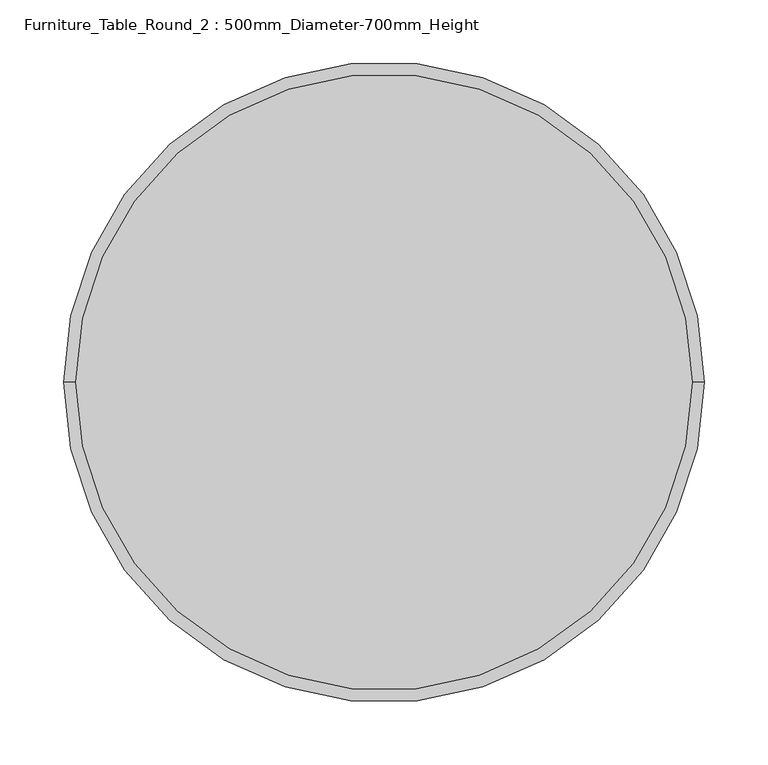
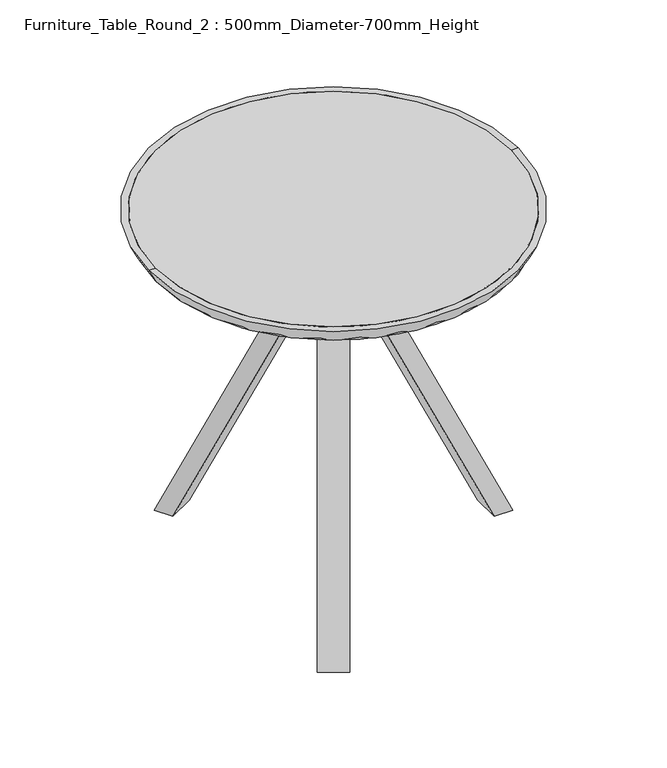
"""IFC4 building model written with IfcOpenShell, lengths in millimetres: furniture geometry, Furniture_Table_Round_2 : 500mm_Diameter-700mm_Height."""

from ifc_helpers import new_model, si_unit, point, frame, frame_2d, origin, origin_2d, place, context, project, spatial, polyline, circle_curve, trimmed, segment, composite_curve, outline, extrude, source, transform, mapped, element, save
from ifc_brep_helpers import plane_surface, revolved_surface, advanced_brep


def furniture_table_round_2_500mm_diameter_700mm_height_9d41381f(model_context):
    return source(origin(), model_context, "Body", "SolidModel", [
        extrude(outline(composite_curve([segment(trimmed(circle_curve(origin_2d(), 241.3), [point((-241.3, 0.0))], [point((241.3, 0.0))], False, "CARTESIAN"), True, "CONTINUOUS"), segment(trimmed(circle_curve(origin_2d(), 241.3), [point((241.3, 0.0))], [point((-241.3, 0.0))], False, "CARTESIAN"), True, "CONTINUOUS")], self_intersect=False)), frame((0.0, 0.0, 482.6), z_axis=(0.0, 0.0, 1.0), x_axis=(1.0, 0.0, 0.0)), (0.0, 0.0, 1.0), 19.05),
        advanced_brep(
        [(241.3, 0.0, 482.6), (-241.3, 0.0, 482.6), (-241.3, 0.0, 501.65), (241.3, 0.0, 501.65), (250.825, 0.0, 501.65), (-250.825, 0.0, 501.65)],
        [
            (0, 1, circle_curve(frame((0.0, 0.0, 482.6), z_axis=(0.0, 0.0, -1.0), x_axis=(-1.0, 0.0, 0.0)), 241.3)),
            (1, 2),
            (2, 3, circle_curve(frame((0.0, 0.0, 501.65), z_axis=(0.0, 0.0, 1.0), x_axis=(-1.0, 0.0, 0.0)), 241.3)),
            (3, 0),
            (4, 5, circle_curve(frame((0.0, 0.0, 501.65), z_axis=(0.0, 0.0, -1.0), x_axis=(-1.0, 0.0, 0.0)), 250.825)),
            (5, 1),
            (0, 4),
            (2, 5),
            (4, 3),
            (1, 0, circle_curve(frame((0.0, 0.0, 482.6), z_axis=(0.0, 0.0, -1.0), x_axis=(1.0, 0.0, 0.0)), 241.3)),
            (3, 2, circle_curve(frame((0.0, 0.0, 501.65), z_axis=(0.0, 0.0, 1.0), x_axis=(1.0, 0.0, 0.0)), 241.3)),
            (5, 4, circle_curve(frame((0.0, 0.0, 501.65), z_axis=(0.0, 0.0, -1.0), x_axis=(1.0, 0.0, 0.0)), 250.825)),
        ],
        [
            revolved_surface(polyline([(-241.3, 0.0, 501.65), (-241.3, 0.0, 482.6)]), (0.0, 0.0, 0.0), (0.0, 0.0, 1.0)),
            revolved_surface(polyline([(-241.3, 0.0, 482.6), (-250.825, 0.0, 501.65)]), (0.0, 0.0, 0.0), (0.0, 0.0, 1.0)),
            plane_surface(frame((0.0, 0.0, 501.65), z_axis=(0.0, 0.0, 1.0), x_axis=(-1.0, 0.0, 0.0))),
            revolved_surface(polyline([(241.3, 0.0, 501.65), (241.3, 0.0, 482.6)]), (0.0, 0.0, 0.0), (0.0, 0.0, 1.0)),
            revolved_surface(polyline([(241.3, 0.0, 482.6), (250.825, 0.0, 501.65)]), (0.0, 0.0, 0.0), (0.0, 0.0, 1.0)),
            plane_surface(frame((0.0, 0.0, 501.65), z_axis=(0.0, 0.0, 1.0), x_axis=(1.0, 0.0, 0.0))),
        ],
        [
            (0, [[1, 2, 3, 4]]),
            (1, [[5, 6, -1, 7]]),
            (2, [[-3, 8, -5, 9]]),
            (3, [[10, -4, 11, -2]]),
            (4, [[12, -7, -10, -6]]),
            (5, [[-11, -9, -12, -8]]),
        ],
    ),
        extrude(outline(composite_curve([segment(polyline([(374.1964885, 32.5393466), (0.0, 207.0300348), (0.0, 232.3753669), (384.9309923, 52.8790974)]), True, "CONTINUOUS"), segment(trimmed(circle_curve(frame_2d((406.4, 98.9195329)), 50.8), [point((384.9309923, 52.8790974))], [point((457.2, 98.9195329))], True, "CARTESIAN"), True, "CONTINUOUS"), segment(polyline([(457.2, 98.9195329), (457.2, 154.8312035), (482.6, 154.8312035), (482.6, 101.6)]), True, "CONTINUOUS"), segment(trimmed(circle_curve(frame_2d((406.4, 101.6)), 76.2), [point((482.6, 101.6))], [point((374.1964885, 32.5393466))], False, "CARTESIAN"), True, "CONTINUOUS")], self_intersect=False)), frame((0.0, -19.05, 0.0), z_axis=(0.0, 1.0, 0.0), x_axis=(0.0, 0.0, 1.0)), (0.0, 0.0, 1.0), 38.1),
        extrude(outline(composite_curve([segment(trimmed(circle_curve(frame_2d((412.8801427, -76.2)), 76.2), [point((412.8801427, 0.0))], [point((481.9407961, -108.4035115))], False, "CARTESIAN"), True, "CONTINUOUS"), segment(polyline([(481.9407961, -108.4035115), (459.4443174, -156.6473658), (436.4240996, -145.9128619), (460.0533926, -95.2396796)]), True, "CONTINUOUS"), segment(trimmed(circle_curve(frame_2d((414.012957, -73.7706719)), 50.8), [point((460.0533926, -95.2396796))], [point((414.0129571, -22.9706718))], True, "CARTESIAN"), True, "CONTINUOUS"), segment(polyline([(414.0129571, -22.9706718), (-10.7114002, -22.9706719), (0.0, 0.0), (412.8801427, 0.0)]), True, "CONTINUOUS")], self_intersect=False)), frame((-120.0128014, 169.7682695, 0.0), z_axis=(0.8660254037844397, 0.4999999999999983, 0.0), x_axis=(0.2113091308703442, -0.36599815077065895, 0.9063077870366545)), (0.0, 0.0, 1.0), 38.1),
        extrude(outline(composite_curve([segment(trimmed(circle_curve(frame_2d((412.8801427, -76.2)), 76.2), [point((412.8801427, 0.0))], [point((481.9407961, -108.4035116))], False, "CARTESIAN"), True, "CONTINUOUS"), segment(polyline([(481.9407961, -108.4035116), (459.4443174, -156.6473658), (436.4240996, -145.9128619), (460.0533926, -95.2396796)]), True, "CONTINUOUS"), segment(trimmed(circle_curve(frame_2d((414.012957, -73.7706719)), 50.8), [point((460.0533926, -95.2396796))], [point((414.0129571, -22.9706718))], True, "CARTESIAN"), True, "CONTINUOUS"), segment(polyline([(414.0129571, -22.9706718), (-10.7114002, -22.9706719), (0.0, 0.0), (412.8801427, 0.0)]), True, "CONTINUOUS")], self_intersect=False)), frame((-87.0172335, -188.8182695, 0.0), z_axis=(-0.8660254037844366, 0.5000000000000038, 0.0), x_axis=(0.21130913087034656, 0.3659981507706578, 0.9063077870366544)), (0.0, 0.0, 1.0), 38.1),
        extrude(outline(composite_curve([segment(trimmed(circle_curve(origin_2d(), 31.7871474), [point((-31.7871474, 0.0))], [point((31.7871474, 0.0))], False, "CARTESIAN"), True, "CONTINUOUS"), segment(trimmed(circle_curve(origin_2d(), 31.7871474), [point((31.7871474, 0.0))], [point((-31.7871474, 0.0))], False, "CARTESIAN"), True, "CONTINUOUS")], self_intersect=False)), frame((0.0, 0.0, 381.0), z_axis=(0.0, 0.0, 1.0), x_axis=(1.0, 0.0, 0.0)), (0.0, 0.0, 1.0), 50.8),
    ])


if __name__ == "__main__":
    model = new_model("IFC4")
    model_context = context("Model", 3, world=origin())
    ifc_project = project(units=[si_unit("LENGTHUNIT", "METRE", prefix="MILLI")], contexts=[model_context])
    site = spatial("IfcSite", under=ifc_project)
    building = spatial("IfcBuilding", under=site)
    placement = place(None, origin())
    furniture_table_round_2_500mm_diameter_700mm_height_shape = furniture_table_round_2_500mm_diameter_700mm_height_9d41381f(model_context)
    element("IfcFurniture", 1, ObjectType="Furniture_Table_Round_2 : 500mm_Diameter-700mm_Height", at=placement, inside=building, context=model_context, shape_type="MappedRepresentation", body=[
        mapped(furniture_table_round_2_500mm_diameter_700mm_height_shape, transform((0.0, 0.0, 0.0), x_axis=(1.0, 0.0, 0.0), y_axis=(0.0, 1.0, 0.0), z_axis=(0.0, 0.0, 1.0))),
    ])
    save(model, "model.ifc")

# Revit data of these elements
# Type "Furniture_Table_Round_2 : 500mm_Diameter-700mm_Height"
#   Keynote = "N"
#   Material Frame = Wood - Birch
#   Material Top = Laminate - Ivory, Matte
#   Default Elevation = 0
#   Assembly Code = ""
# Element 1 (IfcFurniture, "Furniture_Table_Round_2 : 500mm_Diameter-700mm_Height")
#   Materials on its faces: "Wood - Birch", "Laminate - Ivory, Matte"
# Materials
#   "Wood - Birch": class "Wood", colour RGB 213 164 103, transparency 0
#   "Laminate - Ivory, Matte": colour RGB 247 247 239, transparency 0
